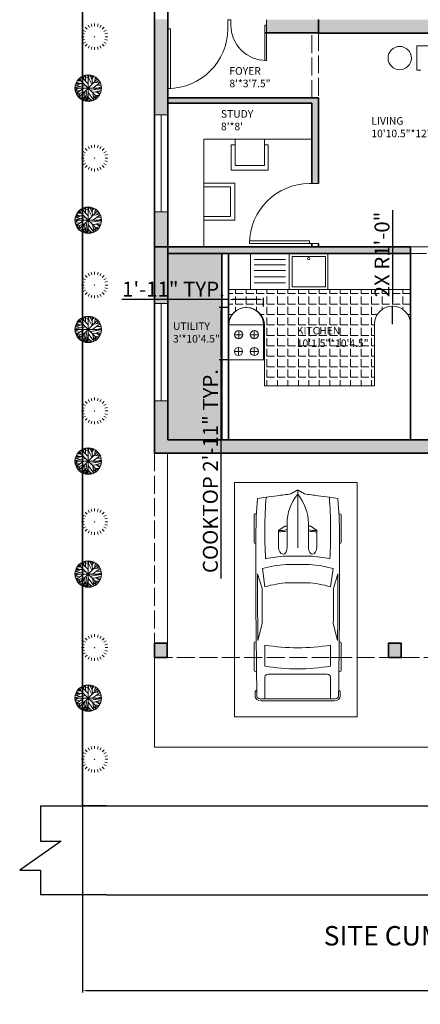
# Model space of a CAD drawing. Units: inches. Extents: x 2852 to 3654, y 1718 to 3031.
# Tile 1 of 5: x 2852 to 3120, y 1718 to 2376. Entities that reach past the tile are written whole.
import ezdxf

# ---------------------------------------------------------------- set-up
doc = ezdxf.new("R2010")
doc.units = ezdxf.units.IN
doc.linetypes.add('ACAD_ISO02W100', pattern=[15, 12, -3])
for name, color, linetype, lineweight in [('A-ANNO-DIMS', 2, 'Continuous', 18), ('A-ANNO-TITL', 7, 'Continuous', 35), ('A-AREA-IDEN', 7, 'Continuous', 18), ('A-COLS', 7, 'Continuous', 35), ('A-COLS-PATT', 8, 'Continuous', 13), ('A-DOOR', 140, 'Continuous', 18), ('A-EQPM', 210, 'Continuous', 18), ('A-FLOR-CASE', 210, 'Continuous', 18), ('A-FLOR-FIXT', 9, 'Continuous', 18), ('A-FLOR-PATT', 52, 'Continuous', 13), ('A-ROOF-OVHD', 140, 'ACAD_ISO02W100', 18), ('A-WALL-OVHD', 140, 'ACAD_ISO02W100', 18), ('A-WALL-PATT', 12, 'Continuous', 13), ('C-PKNG', 8, 'Continuous', 18), ('C-PKNG-VEHI', 140, 'Continuous', 13), ('C-PROP', 7, 'Continuous', 35), ('C-ROAD', 7, 'Continuous', 25), ('fur', 210, 'Continuous', 18), ('tree', 74, 'Continuous', 13), ('wall', 12, 'Continuous', 35), ('window', 140, 'Continuous', 18)]:
    doc.layers.add(name, color=color, linetype=linetype, lineweight=lineweight)
doc.styles.get("Standard").update_dxf_attribs({"font": 'arial.ttf'})
doc.dimstyles.new('ISO-25', dxfattribs={"dimtxt": 10, "dimasz": 2.5, "dimexe": 1.25, "dimexo": 0.625, "dimtad": 1, "dimdec": 0, "dimlunit": 4, "dimtxsty": 'Standard', "dimcen": 2.5, "dimadec": 0, "dimazin": 0, "dimtfac": 1, "dimtdec": 0, "dimtmove": 0, "dimatfit": 3, "dimfxl": 1, "dimarcsym": 0})
pattern_1 = [(0, (0, 0), (0, 6.985), [5.08, -1.905]), (90, (0, 0), (-6.985, 4e-16), [5.08, -1.905])]

# ---------------------------------------------------------------- blocks, each defined once
blk = doc.blocks.new('*U2')
for p, q in [((0, 0), (0, -6)), ((40, 0), (40, -6))]:
    blk.add_line(p, q)
blk.add_lwpolyline([(0, 0), (0, 40), (1.75, 40), (1.75, 0)], close=True)
blk.add_arc((0, 0), 40, 0, 90)
blk = doc.blocks.new('*U6')
for p, q in [((21.1, 37.41), (21.1, 36.83)), ((46.55, 38.89), (22.35, 38.89)), ((47.8, 37.39), (47.8, 37.41)), ((87.99, 31.87), (74.76, 35.92)), ((134.31, 35.6), (119.29, 31.78)), ((135.45, 37.07), (135.45, 37.41)), ((136.7, 38.89), (160.9, 38.89)), ((162.15, 37.41), (162.15, 36.77)), ((70.03, 31.54), (86.41, 29.35)), ((138.42, 29.35), (157.25, 29.35)), ((186.47, 29.35), (167.01, 29.35)), ((186.47, -33.5), (186.47, 33.5)), ((188.4, -32.76), (188.4, 32.76)), ((164.52, 26.39), (164.52, -26.39)), ((29.77, 9.51), (51.68, 9.51)), ((32.12, 9.51), (32.12, 11.15)), ((32.27, 11.63), (36.13, 17.17)), ((36.13, 17.17), (50.94, 17.17)), ((58.92, -10.77), (58.92, 10.77)), ((66.55, -10.53), (66.55, 10.53)), ((186.47, -10.53), (186.47, 10.53)), ((3.27, 6.13), (0.1, 0.41)), ((82.74, 8.5), (82.74, -8.5)), ((0, 0), (51.68, 0)), ((0.1, -0.41), (3.27, -6.13)), ((29.77, -9.51), (51.68, -9.51)), ((32.12, -9.51), (32.12, -11.15)), ((32.27, -11.63), (36.13, -17.17)), ((36.13, -17.17), (50.94, -17.17)), ((86.41, -29.35), (70.03, -31.54)), ((87.99, -31.87), (74.76, -35.92)), ((134.31, -35.6), (119.29, -31.78)), ((157.25, -29.35), (138.42, -29.35)), ((167.01, -29.35), (186.47, -29.35)), ((21.1, -37.41), (21.1, -36.83)), ((46.55, -38.89), (22.35, -38.89)), ((47.8, -37.39), (47.8, -37.41)), ((135.45, -37.07), (135.45, -37.41)), ((136.7, -38.89), (160.9, -38.89)), ((162.15, -37.41), (162.15, -36.77))]:
    blk.add_line(p, q)
for centre, major_axis, ratio, start_param, end_param in [((266.03, -27.52), (0, 313.31), 0.842304, 1.367076, 1.39176), ((41.19, -490.86), (0, 528.23), 0.842304, 0.00281, 0.075598), ((22.35, 37.41), (0, -1.48), 0.842304, 3.141593, 4.712389), ((64.48, -10555.62), (0, 10593.03), 0.842304, -0.013397, 0.002797), ((46.55, 37.41), (0, 1.48), 0.842304, -1.570796, 0), ((64.48, -10555.62), (0, -10591.55), 0.842304, 3.133765, 3.140441), ((136.7, 37.41), (0, -1.48), 0.842304, 3.141593, 4.712389), ((160.9, 37.41), (0, 1.48), 0.842304, -1.570796, 0), ((180.63, 35.84), (0, 2.22), 0.842304, -0.013017, 1.249894), ((64.48, -10556.36), (0, 10595.31), 0.842304, -0.013397, -0.013017), ((183.98, 33.5), (0, -2.96), 0.842304, 1.570796, 3.128196), ((183.98, 32.76), (0, -5.25), 0.842304, 1.570796, 3.128196), ((259.18, -27.52), (0, -305.3), 0.842304, 4.528606, 4.561838), ((37.47, -593.96), (0, -623.33), 0.842304, 3.096046, 3.200911), ((134.4, 5.39), (0, -89.78), 0.842304, 4.449482, 4.652344), ((135.29, 5.39), (0, 81.77), 0.842304, 1.245306, 1.50788), ((149.6, 2.8), (0, -79.58), 0.842304, 4.372215, 4.640744), ((95.79, -3666.35), (0, -3698.24), 0.842304, 3.134049, 3.144098), ((17.08, 0), (0, 147.02), 0.842304, 4.511394, 4.913384), ((35.91, 0), (0, 147.02), 0.842304, 4.511394, 4.913384), ((167.01, 26.39), (0, 2.96), 0.842304, 0, 1.570796), ((-204.49, 52.4), (0, -250.96), 0.842304, 1.385369, 1.434372), ((29.77, -46.66), (0, 56.17), 0.842304, 0, 0.590319), ((32.75, 11.15), (0, 0.74), 0.842304, 0.879714, 1.570796), ((13.04, 17.01), (0, 27.42), 0.842304, 4.435146, 4.718221), ((14.2, 17.01), (0, 27.42), 0.842304, 4.435146, 4.718221), ((50.79, 13.34), (6.34, -0.36), 0.603834, -1.395552, 1.581315), ((0.62, 0), (0, -0.74), 0.842304, 4.131459, 5.293319), ((-204.49, -52.4), (0, 250.96), 0.842304, -1.434372, -1.385369), ((29.77, 46.66), (0, 56.17), 0.842304, 2.551274, 3.141593), ((149.6, -2.8), (0, -79.58), 0.842304, -1.499151, -1.230623), ((32.75, -11.15), (0, -0.74), 0.842304, 4.712389, 5.403472), ((13.04, -17.01), (0, -27.42), 0.842304, 1.564964, 1.848039), ((14.2, -17.01), (0, -27.42), 0.842304, 1.564964, 1.848039), ((134.4, -5.39), (0, -89.78), 0.842304, -1.510751, -1.307889), ((135.29, -5.39), (0, -81.77), 0.842304, -1.50788, -1.245306), ((259.18, 27.52), (0, 305.3), 0.842304, 1.721348, 1.754579), ((167.01, -26.39), (0, -2.96), 0.842304, 4.712389, 6.283185), ((266.03, 27.52), (0, 313.31), 0.842304, 1.749832, 1.774517), ((37.47, 593.96), (0, -623.33), 0.842304, -0.059319, 0.045547), ((95.79, 3666.35), (0, -3698.24), 0.842304, -0.002505, 0.007544), ((183.98, -33.5), (0, 2.96), 0.842304, 3.15499, 4.712389), ((183.98, -32.76), (0, -5.25), 0.842304, 0.013397, 1.570796), ((41.19, 490.86), (0, -528.23), 0.842304, -0.075598, -0.00281), ((22.35, -37.41), (0, 1.48), 0.842304, 1.570796, 3.141593), ((64.48, 10555.62), (0, 10593.03), 0.842304, 3.138796, 3.15499), ((46.55, -37.41), (0, -1.48), 0.842304, 0, 1.570796), ((64.48, 10555.62), (0, -10591.55), 0.842304, 0.001152, 0.007828), ((136.7, -37.41), (0, -1.48), 0.842304, -1.570796, 0), ((160.9, -37.41), (0, 1.48), 0.842304, 3.141593, 4.712389), ((180.63, -35.84), (0, -2.22), 0.842304, -1.249894, 0.013017), ((64.48, 10556.36), (0, 10595.31), 0.842304, 3.15461, 3.15499)]:
    blk.add_ellipse(centre, major_axis=major_axis, ratio=ratio, start_param=start_param, end_param=end_param)
at = {"extrusion": (0, 0, -1)}
blk.add_ellipse((50.79, -13.34), major_axis=(6.34, 0.36), ratio=0.603834, start_param=-1.395552, end_param=1.581315, dxfattribs=at)
blk = doc.blocks.new('*U10')
for p, q in [((-40.1797, 44.558), (-36.4825, 43.2038)), ((-37.0107, 47.0408), (-35.25, 35.5298)), ((-32.6092, 50.4264), (-23.2782, 23.5674)), ((-31.2008, 51.1035), (-0.2149, 20.1818)), ((-26.4472, 46.5894), (-26.2712, 53.8116)), ((-22.0458, 42.0753), (-16.5881, 57.6486)), ((-21.1656, 55.8436), (-0.0388, 45.0094)), ((-12.5388, 54.9406), (-7.9613, 59.4546)), ((-12.3627, 32.1443), (-12.5388, 58.7776)), ((-5.3205, 59.6806), (16.5105, 16.7963)), ((2.426, 54.9406), (-1.4472, 59.9056)), ((0, 59.9996), (0, -60)), ((0.4894, 48.6208), (3.6584, 59.6806)), ((18.2711, 35.5298), (5.419, 59.6806)), ((9.8203, 51.5549), (12.8133, 58.5516)), ((19.6795, 19.5047), (16.3344, 57.6486)), ((17.0387, 51.1035), (23.2006, 55.1666)), ((17.7429, 43.6552), (25.4894, 54.2636)), ((31.6513, 50.8778), (30.2429, 30.5643)), ((31.1232, 42.5267), (35.8767, 48.1693)), ((-59.7219, 2.8025), (-12.0106, 12.0565)), ((-32.2571, 20.6333), (-59.1937, 9.348)), ((-58.6656, 12.7336), (-35.9543, 7.5424)), ((-57.081, 17.9248), (-47.0458, 14.7649)), ((-56.0247, 20.859), (-20.8134, 20.859)), ((-54.7923, 24.4702), (-47.75, 21.0847)), ((-54.6162, -24.7335), (-20.2853, 0.0941)), ((-53.2078, 27.4044), (-40.1797, 20.859)), ((-49.8627, 32.8214), (-32.7853, 32.8214)), ((-45.8134, 38.2383), (-40.5318, 33.0471)), ((-43.8768, 36.4326), (-44.405, 40.2696)), ((42, 42), (-42, -42)), ((42, -42), (-42, 42)), ((54.3626, 25.3731), (20.9119, 0.3198)), ((23.3767, 23.3417), (53.3063, 27.4044)), ((29.3626, -6.6771), (59.4682, 7.091)), ((36.2288, 25.1474), (48.9049, 35.0784)), ((37.1091, 37.1098), (46.6161, 37.5612)), ((38.5175, 13.4107), (58.2359, 13.6364)), ((-60, 0), (60, 0)), ((-59.7219, -4.8714), (-54.2641, -6.6771)), ((-45.2853, -0.1316), (-59.0177, -10.0627)), ((-58.4895, -12.3197), (-36.4825, -11.6426)), ((-57.081, -18.4138), (-45.2853, -17.9624)), ((-52.6797, -18.188), (-55.4966, -22.0251)), ((-53.2078, -27.442), (-16.7641, -16.6081)), ((-38.9472, -29.0219), (-51.4472, -30.6018)), ((-47.2219, -19.3166), (-50.2148, -26.3135)), ((-46.5177, -30.1504), (-49.5106, -33.536)), ((-32.4331, -32.4075), (-48.1021, -35.5674)), ((-43.7008, -34.6645), (-46.6937, -37.373)), ((-35.9543, -22.4765), (-44.0529, -40.5329)), ((-24.6867, -37.8244), (-38.7712, -45.7241)), ((-26.2712, -43.9185), (-34.7219, -48.6583)), ((-19.9331, -20.2194), (-28.5599, -52.721)), ((-14.6515, -36.2445), (-27.6797, -52.9467)), ((-14.8275, -15.0282), (-14.6515, -57.6865)), ((-14.6515, -32.1818), (-3.912, -59.4922)), ((-10.074, -10.0627), (-2.5036, -59.7178)), ((-6.2008, -36.2445), (17.919, -57.0094)), ((-0.0388, -19.0909), (25.8415, -53.8495)), ((9.2922, -9.1598), (59.6443, -2.8401)), ((18.6232, -18.6394), (26.7218, -53.3981)), ((18.7992, -18.6394), (57.3556, -17.2853)), ((22.8485, -36.4702), (35.3485, -48.4326)), ((26.3697, -18.4138), (58.9401, -9.8369)), ((30.419, -30.1504), (32.3556, -50.0125)), ((31.4753, -31.279), (49.6091, -33.3103)), ((38.1654, -18.188), (52.426, -29.0219)), ((41.5105, -32.6332), (46.088, -38.0501)), ((45.9119, -24.0564), (55.595, -22.2508)), ((-14.6515, -47.3041), (-25.0388, -54.3009)), ((-21.5177, -45.4984), (-19.9331, -56.1065)), ((-8.4895, -47.5298), (-11.4825, -58.5893)), ((-6.3768, -52.721), (-9.3698, -58.815)), ((8.4119, -53.1724), (3.8344, -59.4922)), ((5.9471, -46.6269), (10.5246, -58.5893)), ((24.7852, -44.8213), (23.0246, -54.978))]:
    blk.add_line(p, q)
blk.add_circle((0, 0), 60)
blk = doc.blocks.new('*U9')
for p, q in [((-25.024, 42.079), (-31.077, 52.563)), ((-13.435, 46.72), (-16.606, 58.557)), ((-1.077, 60.601), (-1.077, 48.601)), ((11.28, 46.72), (14.452, 58.557)), ((22.87, 42.079), (28.923, 52.563)), ((-61.077, 0.601), (-49.077, 0.601)), ((-47.5, 13.04), (-59.033, 16.131)), ((-42.564, 24.554), (-53.039, 30.601)), ((-34.93, 34.454), (-43.503, 43.028)), ((32.776, 34.454), (41.349, 43.028)), ((40.409, 24.554), (50.884, 30.601)), ((45.346, 13.04), (56.878, 16.131)), ((58.923, 0.601), (46.923, 0.601)), ((-47.5, -11.837), (-59.033, -14.928)), ((-42.564, -23.351), (-53.039, -29.399)), ((-34.93, -33.251), (-43.503, -41.825)), ((-25.024, -40.876), (-31.077, -51.36)), ((22.87, -40.876), (28.923, -51.36)), ((32.776, -33.251), (41.349, -41.825)), ((40.409, -23.351), (50.884, -29.399)), ((45.346, -11.837), (56.878, -14.928)), ((-13.435, -45.517), (-16.606, -57.354)), ((-1.077, -59.399), (-1.077, -47.399)), ((11.28, -45.517), (14.452, -57.354))]:
    blk.add_line(p, q)
blk.add_lwpolyline([(-1.908, 0.978), (-2.67, -0.978), (0, 0)], close=True)
blk = doc.blocks.new('COOKTOP-4-BURNER')
for p, q in [((8.84, 29.44), (3.38, 29.44)), ((6.11, 32.18), (6.11, 26.71)), ((6.11, 26.71), (6.11, 29.44)), ((6.11, 29.44), (8.84, 29.44)), ((19.4, 29.44), (13.94, 29.44)), ((16.67, 32.18), (16.67, 26.71)), ((16.67, 26.71), (16.67, 29.44)), ((16.67, 29.44), (19.4, 29.44)), ((6.11, 20.96), (6.11, 15.5)), ((16.52, 20.96), (16.52, 15.5)), ((8.84, 18.23), (3.38, 18.23)), ((6.11, 15.5), (6.11, 18.23)), ((6.11, 18.23), (8.84, 18.23)), ((19.25, 18.23), (13.79, 18.23)), ((16.52, 15.5), (16.52, 18.23)), ((16.52, 18.23), (19.25, 18.23))]:
    blk.add_line(p, q)
blk.add_lwpolyline([(0, 35.06), (23.09, 35.06), (23.09, 11.55), (0, 11.55)], close=True)
for centre in [(6.11, 29.44), (16.67, 29.44), (6.11, 18.23), (16.52, 18.23)]:
    blk.add_circle(centre, 2.73)
blk.add_arc((11.55, 11.55), 11.55, 180, 0)
blk = doc.blocks.new('ROAD-BREAK')
for p, q in [((13.81, 59.39), (13.81, 35.82)), ((27.65, 35.82), (12.74, 25.36)), ((13.81, 35.82), (27.65, 35.82)), ((12.74, 25.36), (0, 16.42)), ((0, 16.42), (13.81, 16.42)), ((13.81, 16.42), (13.81, 0))]:
    blk.add_line(p, q)
blk = doc.blocks.new('PARKING-STALL')
blk.add_lwpolyline([(0, 156.52), (82.03, 156.52), (82.03, 0), (0, 0)], close=True)
blk = doc.blocks.new('*D37')
at = {"layer": 'A-ANNO-DIMS', "color": 0, "lineweight": -2, "transparency": 16777216}
for p, q in [((2991.43, 2184.07), (2985.55, 2184.07)), ((2986.8, 2181.57), (2986.8, 2151.51)), ((2991.43, 2149.01), (2985.55, 2149.01)), ((2986.8, 2149.01), (2986.8, 2002.92))]:
    blk.add_line(p, q, dxfattribs=at)
at = {"layer": 'A-ANNO-DIMS', "color": 0, "lineweight": 100, "transparency": 16777216}
for points in [[(2986.38, 2181.57), (2987.22, 2181.57), (2986.8, 2184.07)], [(2986.38, 2151.51), (2987.22, 2151.51), (2986.8, 2149.01)]]:
    blk.add_solid(points, dxfattribs=at)
at = {"layer": 'Defpoints', "color": 0, "lineweight": 100, "transparency": 16777216}
for p in [(2992.06, 2184.07), (2986.8, 2149.01), (2992.06, 2149.01)]:
    blk.add_point(p, dxfattribs=at)
at = {"layer": 'A-ANNO-DIMS', "color": 0, "transparency": 16777216, "insert": (2981, 2074.71), "char_height": 10, "attachment_point": 5, "rotation": 90}
blk.add_mtext('COOKTOP 2\'-11" TYP.', dxfattribs=at)
blk = doc.blocks.new('*D38')
at = {"layer": 'A-ANNO-DIMS', "color": 0, "lineweight": -2, "transparency": 16777216}
for p, q in [((2992.06, 2189.33), (2920.53, 2189.33)), ((2992.06, 2184.69), (2992.06, 2190.58)), ((3012.65, 2189.33), (2994.56, 2189.33)), ((3015.15, 2184.69), (3015.15, 2190.58))]:
    blk.add_line(p, q, dxfattribs=at)
at = {"layer": 'A-ANNO-DIMS', "color": 0, "lineweight": 100, "transparency": 16777216}
for points in [[(2994.56, 2189.74), (2994.56, 2188.91), (2992.06, 2189.33)], [(3012.65, 2189.74), (3012.65, 2188.91), (3015.15, 2189.33)]]:
    blk.add_solid(points, dxfattribs=at)
at = {"layer": 'Defpoints', "color": 0, "lineweight": 100, "transparency": 16777216}
for p in [(2992.06, 2189.33), (2992.06, 2184.07), (3015.15, 2184.07)]:
    blk.add_point(p, dxfattribs=at)
at = {"layer": 'A-ANNO-DIMS', "color": 0, "transparency": 16777216, "insert": (2955.04, 2194.98), "char_height": 10, "attachment_point": 5}
blk.add_mtext('1\'-11" TYP.', dxfattribs=at)
blk = doc.blocks.new('*D39')
at = {"layer": 'A-ANNO-DIMS', "color": 0, "lineweight": -2, "transparency": 16777216}
for p, q in [((2894.37, 1850.19), (2894.37, 1726.13)), ((3510.95, 1850.19), (3510.95, 1726.13)), ((2896.87, 1727.38), (3508.45, 1727.38))]:
    blk.add_line(p, q, dxfattribs=at)
at = {"layer": 'A-ANNO-DIMS', "color": 0, "lineweight": 100, "transparency": 16777216}
for points in [[(2896.87, 1727.79), (2896.87, 1726.96), (2894.37, 1727.38)], [(3508.45, 1727.79), (3508.45, 1726.96), (3510.95, 1727.38)]]:
    blk.add_solid(points, dxfattribs=at)
at = {"layer": 'Defpoints', "color": 0, "lineweight": 100, "transparency": 16777216}
for p in [(2894.37, 1850.82), (3510.95, 1850.82), (3510.95, 1727.38)]:
    blk.add_point(p, dxfattribs=at)
at = {"layer": 'A-ANNO-DIMS', "color": 0, "transparency": 16777216, "insert": (3202.66, 1733.17), "char_height": 10, "attachment_point": 5}
blk.add_mtext('51\'-4 1/2"', dxfattribs=at)
blk = doc.blocks.new('*D41')
at = {"layer": 'A-ANNO-DIMS', "color": 0, "lineweight": -2, "transparency": 16777216}
for p, q in [((3101.37, 2248.99), (3101.37, 2187.43)), ((3101.37, 2172.93), (3101.37, 2184.93))]:
    blk.add_line(p, q, dxfattribs=at)
at = {"layer": 'A-ANNO-DIMS', "color": 0, "lineweight": 100, "transparency": 16777216}
blk.add_solid([(3100.95, 2187.43), (3101.78, 2187.43), (3101.37, 2184.93)], dxfattribs=at)
at = {"layer": 'Defpoints', "color": 0, "lineweight": 100, "transparency": 16777216}
for p in [(3101.37, 2184.93), (3101.37, 2172.93)]:
    blk.add_point(p, dxfattribs=at)
at = {"layer": 'A-ANNO-DIMS', "color": 0, "transparency": 16777216, "insert": (3095.64, 2219.46), "char_height": 10, "attachment_point": 5, "rotation": 89.99977}
blk.add_mtext('2X R1\'-0"', dxfattribs=at)

msp = doc.modelspace()

# ---------------------------------------------------------------- hatches: boundary and pattern name
at = {"layer": 'A-COLS-PATT'}
h = msp.add_hatch(color=256, dxfattribs=at)
h.dxf.hatch_style = 1
h.paths.add_polyline_path([(2950.9, 1959.59), (2942.37, 1959.59), (2942.37, 1950.07), (2950.9, 1950.07)])
h.paths.add_polyline_path([(3107.14, 1959.59), (3098.61, 1959.59), (3098.61, 1950.07), (3107.14, 1950.07)])
h.paths.add_polyline_path([(3238.77, 1959.59), (3230.24, 1959.59), (3230.24, 1950.07), (3238.77, 1950.07)])
h.paths.add_polyline_path([(3429.87, 1959.59), (3421.34, 1959.59), (3421.34, 1950.07), (3429.87, 1950.07)])
at = {"layer": 'A-FLOR-PATT'}
h = msp.add_hatch(dxfattribs=at)
h.set_pattern_fill('ANGLE', color=256)
h.set_pattern_definition(pattern_1)
h.paths.add_polyline_path([(3248.45, 2849.58), (3188.45, 2849.58), (3188.45, 2844.77), (3196.45, 2844.77), (3196.45, 2842.27), (3196.95, 2842.27), (3196.95, 2844.27), (3197.95, 2844.27), (3197.95, 2841.27), (3196.45, 2841.27), (3196.45, 2838.27), (3202.45, 2840.27, -0.501317), (3221.31, 2835.31, -0.132891), (3221.31, 2833.22, -0.501323), (3202.45, 2828.27), (3196.45, 2830.27), (3196.45, 2823.77), (3188.45, 2823.77), (3188.45, 2783.69), (3215.78, 2783.69), (3215.78, 2783.73, -0.401453), (3244.71, 2813.96), (3244.71, 2813.99), (3246.03, 2813.99), (3246.03, 2783.69), (3248.45, 2783.69)])
h.paths.add_polyline_path([(3420.95, 2714.69), (3324.42, 2714.69), (3324.42, 2691.18, -1), (3301.33, 2691.18), (3301.33, 2638.19), (3420.95, 2638.19)])
h.paths.add_polyline_path([(3059.57, 2647.05, -0.132891), (3061.66, 2647.05, -0.501323), (3066.62, 2628.19), (3064.62, 2622.19), (3071.12, 2622.19), (3071.12, 2614.19), (3084.95, 2614.19), (3084.95, 2678.69), (3040.14, 2678.69), (3040.14, 2677.19), (3040.14, 2637.19), (3038.39, 2637.19), (3038.39, 2637.23, -0.401453), (3000.14, 2677.19), (3000.14, 2678.69), (2994.25, 2678.69), (2994.25, 2614.19), (3050.12, 2614.19), (3050.12, 2622.19), (3052.62, 2622.19), (3052.62, 2622.69), (3050.62, 2622.69), (3050.62, 2623.69), (3053.62, 2623.69), (3053.62, 2622.19), (3056.62, 2622.19), (3054.62, 2628.19, -0.501317)])
h.paths.add_polyline_path([(3252.95, 2533.88, -0.400409), (3223.79, 2561.89), (3223.76, 2561.89), (3223.76, 2563.17), (3252.95, 2563.17), (3252.95, 2565.48), (3192.95, 2565.48), (3192.95, 2500.92), (3252.95, 2500.92)])
h.paths.add_polyline_path([(3248.45, 2338.72), (3188.45, 2338.72), (3188.45, 2271.48), (3248.45, 2271.48), (3248.45, 2273.69)])
h.paths.add_polyline_path([(3390.34, 2273.69), (3312.95, 2273.69), (3312.95, 2224.19), (3390.34, 2224.19)])
h.paths.add_polyline_path([(3365.33, 2231.19), (3382.33, 2231.19, -0.5), (3383.33, 2230.19), (3383.33, 2226.19, -0.5), (3382.33, 2225.19), (3365.33, 2225.19, -0.5), (3364.33, 2226.19), (3364.33, 2230.19, -0.5)], flags=16)
h.paths.add_polyline_path([(3372.19, 2255.72, -0.215004), (3375.48, 2255.72, -0.48008), (3377.83, 2238.19), (3369.83, 2238.19, -0.48008)], flags=16)
h.paths.add_polyline_path([(2987.37, 2220.07), (2951.37, 2220.07), (2951.37, 2095.57), (2987.37, 2095.57)])
h = msp.add_hatch(dxfattribs=at)
h.set_pattern_fill('ANGLE', color=256)
h.set_pattern_definition(pattern_1)
h.paths.add_polyline_path([(3113.37, 2172.93), (3113.37, 2196.07), (2991.87, 2196.07), (2991.87, 2172.07, -1), (3015.87, 2172.07), (3015.87, 2146.36), (3015.87, 2131.57), (3089.37, 2131.57), (3089.37, 2138.18), (3089.37, 2172.93, -1)])
at = {"layer": 'A-WALL-PATT'}
h = msp.add_hatch(color=256, dxfattribs=at)
h.dxf.hatch_style = 1
h.paths.add_polyline_path([(2952.95, 2875.19), (2957.35, 2875.19), (2957.35, 2877.98), (2957.35, 2884.19), (2943.95, 2884.19), (2942.37, 2884.19), (2942.37, 2849.42), (2952.95, 2849.42)])
h.paths.add_polyline_path([(2952.95, 2706.39), (2952.95, 2749.45), (2942.37, 2749.45), (2942.37, 2667.89), (2952.95, 2667.89), (2952.95, 2678.69), (3000.14, 2678.69), (3000.14, 2683.19), (2952.95, 2683.19)])
h.paths.add_polyline_path([(2951.37, 2609.69), (3089.45, 2609.69), (3089.45, 2683.19), (3089.45, 2685.28), (3084.95, 2685.28), (3084.95, 2683.19), (3084.95, 2614.19), (2952.95, 2614.19), (2952.95, 2625.26), (2942.37, 2625.26), (2942.37, 2588.19), (2951.37, 2588.19)])
h.paths.add_polyline_path([(2951.37, 2506.48), (2951.37, 2523.26), (2942.37, 2523.26), (2942.37, 2465.69), (2951.37, 2465.69), (2951.37, 2466.48)])
h.paths.add_polyline_path([(2951.37, 2367.57), (2951.37, 2370.4), (2951.37, 2376.57), (2942.37, 2376.57), (2942.37, 2312.8), (2951.37, 2312.8), (2951.37, 2320.57), (2951.37, 2324.07)])
h.paths.add_polyline_path([(3051.87, 2324.07), (3047.37, 2324.07), (2951.37, 2324.07), (2951.37, 2320.57), (3047.37, 2320.57), (3047.37, 2296.57), (3047.37, 2266.82), (3051.87, 2266.82)])
h.paths.add_polyline_path([(2951.37, 2224.57), (2942.37, 2224.57), (2942.37, 2186.63), (2951.37, 2186.63), (2951.37, 2220.07)])
h.paths.add_polyline_path([(2951.37, 2247.87), (2942.37, 2247.87), (2942.37, 2224.57), (2951.37, 2224.57)])
h.paths.add_polyline_path([(3113.37, 2224.57), (2951.37, 2224.57), (2951.37, 2220.07), (3113.37, 2220.07)])
h.paths.add_polyline_path([(2951.37, 2121.7), (2942.37, 2121.7), (2942.37, 2086.57), (3113.37, 2086.57), (3147.16, 2086.57), (3147.16, 2095.57), (3113.37, 2095.57), (2951.37, 2095.57)])
h.paths.add_polyline_path([(3429.87, 2224.19), (3276.87, 2224.19), (3276.87, 2219.69), (3420.87, 2219.69), (3420.87, 2182.43), (3429.87, 2182.43)])
h.paths.add_polyline_path([(3276.87, 2175.85), (3272.37, 2175.85), (3272.37, 2095.57), (3240.86, 2095.57), (3240.86, 2086.57), (3276.87, 2086.57)])
h.paths.add_polyline_path([(3276.87, 2224.57), (3234.52, 2224.57), (3234.52, 2220.07), (3272.37, 2220.07), (3272.37, 2215.85), (3276.87, 2215.85)])
h = msp.add_hatch(color=256, dxfattribs=at)
h.dxf.hatch_style = 1
h.paths.add_polyline_path([(3188.45, 2266.98), (3183.95, 2266.98), (3183.95, 2224.57), (3183.95, 2220.07), (3205.81, 2220.07), (3205.81, 2224.57), (3188.45, 2224.57)])
h.paths.add_polyline_path([(3188.45, 2367.48), (3183.95, 2367.48), (3183.95, 2266.98), (3188.45, 2266.98), (3188.45, 2271.48)])
h.paths.add_polyline_path([(3051.87, 2376.48), (3017.1, 2376.48), (3017.1, 2372.85), (3017.1, 2367.57), (3047.37, 2367.57), (3051.87, 2367.57), (3051.87, 2372.07)])
h.paths.add_polyline_path([(3197.45, 2376.48), (3197.45, 2460.48), (3225.82, 2460.48), (3225.82, 2469.48), (3188.45, 2469.48), (3188.45, 2376.48), (3051.87, 2376.48), (3051.87, 2372.07), (3051.87, 2367.48), (3197.45, 2367.48)])
h.paths.add_polyline_path([(3257.45, 2410.19), (3257.45, 2469.48), (3247.17, 2469.48), (3247.17, 2460.48), (3248.45, 2460.48), (3248.45, 2376.48), (3218.8, 2376.48), (3218.8, 2367.48), (3257.45, 2367.48)])
h.paths.add_polyline_path([(3257.45, 2367.48), (3252.95, 2367.48), (3252.95, 2278.19), (3257.45, 2278.19)])
h.paths.add_polyline_path([(3420.95, 2278.19), (3308.45, 2278.19), (3308.45, 2273.69), (3420.95, 2273.69)])
h.paths.add_polyline_path([(3257.45, 2527.51), (3257.45, 2533.88), (3252.95, 2533.88), (3252.95, 2469.48), (3257.45, 2469.48)])
h.paths.add_polyline_path([(3257.45, 2609.69), (3259.24, 2609.69), (3259.24, 2614.19), (3252.95, 2614.19), (3227.77, 2614.19), (3227.77, 2611.84), (3227.77, 2609.69), (3252.95, 2609.69), (3252.95, 2563.17), (3253.06, 2563.17), (3257.45, 2563.17)])
h.paths.add_polyline_path([(3196.43, 2614.19), (3188.45, 2614.19), (3188.45, 2569.84), (3188.45, 2469.48), (3192.95, 2469.48), (3192.95, 2565.48), (3252.95, 2565.48), (3252.95, 2569.98), (3192.95, 2569.98), (3192.95, 2609.69), (3196.43, 2609.69), (3196.43, 2611.84)])

# ---------------------------------------------------------------- linework, layer by layer
at = {"layer": 'A-COLS'}
for p, q in [((2942.37, 1959.59), (2942.37, 1950.07)), ((2942.37, 1950.07), (2950.9, 1950.07))]:
    msp.add_line(p, q, dxfattribs=at)
for points in [[(2942.37, 1950.07), (2950.9, 1950.07), (2950.9, 1959.59), (2942.37, 1959.59)], [(3098.61, 1950.07), (3107.14, 1950.07), (3107.14, 1959.59), (3098.61, 1959.59)]]:
    msp.add_lwpolyline(points, close=True, dxfattribs=at)
at = {"layer": 'A-FLOR-CASE'}
for p, q in [((3047.37, 2320.57), (3047.37, 2296.57)), ((2975.37, 2224.57), (2975.37, 2296.57)), ((3047.37, 2296.57), (2975.37, 2296.57)), ((2951.37, 2224.57), (2975.37, 2224.57)), ((2991.87, 2220.07), (2991.87, 2196.07)), ((2991.87, 2196.07), (3113.37, 2196.07)), ((2991.87, 2196.07), (3015.87, 2196.07)), ((2991.87, 2196.07), (2991.87, 2172.07)), ((3113.37, 2196.07), (3089.37, 2196.07)), ((3113.37, 2196.07), (3113.37, 2172.07)), ((3015.87, 2172.07), (3015.87, 2146.36)), ((3089.37, 2172.93), (3089.37, 2138.18)), ((3015.87, 2146.36), (3015.87, 2131.57)), ((3089.37, 2138.18), (3089.37, 2131.57)), ((2991.87, 2095.57), (2991.87, 2131.57)), ((3015.87, 2131.57), (3089.37, 2131.57))]:
    msp.add_line(p, q, dxfattribs=at)
for centre in [(3003.87, 2172.07), (3101.37, 2172.93)]:
    msp.add_arc(centre, 12, 0, 180, dxfattribs=at)
at = {"layer": 'A-FLOR-FIXT'}
for p, q in [((3032.32, 2220.07), (3032.37, 2196.07)), ((3008.97, 2216), (3029.89, 2216)), ((3008.97, 2212.47), (3029.89, 2212.47)), ((3008.97, 2208.72), (3029.89, 2208.72)), ((3008.97, 2204.54), (3029.89, 2204.54)), ((3008.97, 2200.57), (3029.89, 2200.57))]:
    msp.add_line(p, q, dxfattribs=at)
for points in [[(3006.4, 2220.07), (3058.24, 2220.07), (3058.24, 2196.07), (3006.4, 2196.07)], [(3034.29, 2218.15), (3056.71, 2218.15), (3056.71, 2197.78), (3034.29, 2197.78)]]:
    msp.add_lwpolyline(points, close=True, dxfattribs=at)
msp.add_circle((3045.32, 2216.69), 0.817, dxfattribs=at)
at = {"layer": 'A-ROOF-OVHD'}
for p, q in [((2942.37, 2086.57), (2942.37, 1950.07)), ((2942.37, 1950.07), (3429.87, 1950.07))]:
    msp.add_line(p, q, dxfattribs=at)
at = {"layer": 'A-WALL-OVHD'}
msp.add_line((2991.37, 2376.4), (2993.37, 2376.4), dxfattribs=at)
for points in [[(3051.87, 2324.07), (3047.37, 2324.07), (3047.37, 2367.57), (3051.87, 2367.57)], [(3113.37, 2224.57), (3183.95, 2224.57), (3183.95, 2220.07), (3113.37, 2220.07)]]:
    msp.add_lwpolyline(points, close=True, dxfattribs=at)
at = {"layer": 'C-PKNG'}
for p, q in [((2951.02, 2086.57), (2951.02, 1966.37)), ((2951.02, 1966.37), (2951.02, 1959.59)), ((2942.37, 1950.07), (2942.37, 1890.07)), ((3008.96, 1950.07), (3010.43, 1950.07)), ((3059.99, 1950.07), (3067.12, 1950.07)), ((3098.61, 1950.07), (3107.14, 1950.07)), ((2942.37, 1890.07), (3429.87, 1890.07))]:
    msp.add_line(p, q, dxfattribs=at)
at = {"layer": 'C-PROP'}
for p, q in [((2894.37, 1890.07), (2894.37, 2927.69)), ((2894.37, 1890.07), (2894.37, 1850.82)), ((2894.37, 1850.82), (2910.23, 1850.82))]:
    msp.add_line(p, q, dxfattribs=at)
at = {"layer": 'C-ROAD'}
for p, q in [((2866.16, 1850.82), (2910.23, 1850.82)), ((2910.23, 1850.82), (3468.85, 1850.82)), ((2910.23, 1791.43), (2866.16, 1791.43)), ((2910.23, 1791.43), (3468.85, 1791.43))]:
    msp.add_line(p, q, dxfattribs=at)
at = {"layer": 'fur'}
for p, q in [((3117.65, 2342.6), (3117.65, 2358.82)), ((3117.65, 2358.82), (3156.83, 2358.82)), ((3120.33, 2342.6), (3117.65, 2342.6)), ((2996.17, 2292.84), (2993.65, 2292.84)), ((2993.65, 2292.84), (2993.65, 2275.9)), ((3018.41, 2292.84), (3015.91, 2292.84)), ((3018.41, 2275.9), (3018.41, 2292.84)), ((2993.65, 2275.9), (3018.41, 2275.9)), ((2979.1, 2267.16), (2975.37, 2267.16)), ((2996.03, 2267.16), (2979.1, 2267.16)), ((2996.03, 2242.4), (2996.03, 2267.16)), ((2979.1, 2242.4), (2975.37, 2242.4)), ((2979.1, 2242.4), (2996.03, 2242.4))]:
    msp.add_line(p, q, dxfattribs=at)
for points in [[(2996.17, 2296.57), (3015.91, 2296.57), (3015.91, 2278.85), (2996.17, 2278.85)], [(2975.37, 2244.92), (2975.37, 2264.67), (2993.09, 2264.67), (2993.09, 2244.92)]]:
    msp.add_lwpolyline(points, close=True, dxfattribs=at)
msp.add_circle((3106.15, 2350.75), 7.79, dxfattribs=at)
at = {"layer": 'wall'}
for p, q in [((2942.37, 2224.57), (2942.37, 2884.19)), ((2951.37, 2609.69), (2951.37, 2367.57)), ((3051.87, 2372.07), (3051.87, 2376.48)), ((3051.87, 2372.07), (3051.87, 2367.48)), ((2951.37, 2324.07), (2951.37, 2367.57)), ((3016.06, 2367.57), (3047.37, 2367.57)), ((3047.37, 2367.57), (3051.87, 2367.57)), ((3051.87, 2367.48), (3248.45, 2367.48)), ((2951.37, 2324.07), (3047.37, 2324.07)), ((2951.37, 2320.57), (2951.37, 2324.07)), ((3047.37, 2324.07), (3051.87, 2324.07)), ((3051.87, 2324.07), (3051.87, 2266.82)), ((2951.37, 2224.57), (2951.37, 2320.57)), ((2951.37, 2320.57), (3047.37, 2320.57)), ((3047.37, 2320.57), (3047.37, 2266.82)), ((3113.37, 2224.57), (2942.37, 2224.57)), ((2942.37, 2224.57), (2942.37, 2086.57)), ((2951.37, 2220.07), (2951.37, 2224.57)), ((3047.37, 2226.82), (3047.37, 2224.57)), ((3051.87, 2226.82), (3051.87, 2224.57)), ((3113.37, 2224.57), (3113.37, 2095.57)), ((3113.37, 2220.07), (2951.37, 2220.07)), ((2951.37, 2220.07), (2951.37, 2095.57)), ((2987.37, 2220.07), (2987.37, 2095.57)), ((2991.87, 2220.07), (2991.87, 2095.57)), ((3113.37, 2095.57), (3113.37, 2220.07)), ((2951.37, 2095.57), (3113.37, 2095.57)), ((3113.37, 2095.57), (3272.37, 2095.57)), ((2942.37, 2086.57), (3113.37, 2086.57)), ((3113.37, 2086.57), (3276.87, 2086.57))]:
    msp.add_line(p, q, dxfattribs=at)
at = {"layer": 'window'}
for p, q in [((2946.87, 2247.87), (2946.87, 2312.8)), ((2946.87, 2121.7), (2946.87, 2186.63))]:
    msp.add_line(p, q, dxfattribs=at)
for points in [[(2942.37, 2312.8), (2951.37, 2312.8), (2951.37, 2247.87), (2942.37, 2247.87)], [(2942.37, 2186.63), (2951.37, 2186.63), (2951.37, 2121.7), (2942.37, 2121.7)]]:
    msp.add_lwpolyline(points, close=True, dxfattribs=at)

# ---------------------------------------------------------------- block references
at = {"layer": 'A-DOOR', "xscale": -1, "rotation": 180}
msp.add_blockref('*U2', (2951.37, 2370.4), dxfattribs=at)
at = {"layer": 'A-DOOR', "xscale": 0.5931757633417637, "yscale": 0.5931757633417637, "zscale": 0.5931757633417637, "rotation": 180}
msp.add_blockref('*U2', (3017.1, 2372.85), dxfattribs=at)
at = {"layer": 'A-DOOR', "rotation": 90}
msp.add_blockref('*U2', (3045.87, 2226.82), dxfattribs=at)
at = {"layer": 'A-EQPM', "rotation": 180}
msp.add_blockref('COOKTOP-4-BURNER', (3015.15, 2184.07), dxfattribs=at)
at = {"layer": 'C-PKNG'}
msp.add_blockref('PARKING-STALL', (2995.75, 1910.51), dxfattribs=at)
at = {"layer": 'C-PKNG-VEHI', "xscale": 0.7477922120772245, "yscale": 0.7477922120772245, "zscale": 0.7477922120772245, "rotation": 270}
msp.add_blockref('*U6', (3038.04, 2061.92), dxfattribs=at)
at = {"layer": 'C-ROAD'}
msp.add_blockref('ROAD-BREAK', (2852.35, 1791.43), dxfattribs=at)
at = {"layer": 'tree', "xscale": 0.1480989313836924, "yscale": 0.1480989313836924, "zscale": 0.1480989313836924}
for name, p in [('*U9', (2902.57, 2364.95)), ('*U10', (2898.14, 2330.64)), ('*U9', (2902.57, 2283.83)), ('*U10', (2898.14, 2242.32)), ('*U9', (2902.57, 2198.97)), ('*U10', (2898.14, 2169.41)), ('*U9', (2902.57, 2114.8)), ('*U10', (2898.14, 2081.35)), ('*U9', (2902.57, 2040.77)), ('*U10', (2898.14, 2005.87)), ('*U9', (2902.57, 1956.61)), ('*U10', (2898.14, 1922.97)), ('*U9', (2902.57, 1881.94))]:
    msp.add_blockref(name, p, dxfattribs=at)

# ---------------------------------------------------------------- texts
at = {"layer": 'A-ANNO-TITL', "insert": (3055.38, 1770.57), "char_height": 12.998, "attachment_point": 1}
msp.add_mtext_dynamic_manual_height_columns('SITE CUM GROUND FLOOR PLAN', width=2588.4992, gutter_width=64.99, heights=[0], dxfattribs=at)
at = {"layer": 'A-AREA-IDEN', "attachment_point": 1}
for s, insert, char_height in [('FOYER\\P8\'*3\'7.5"', (2992.41, 2344.69), 5.041), ("STUDY\\P8'*8'", (2986.79, 2315.94), 5.041), ('LIVING\\P10\'10.5"*12\'', (3087.23, 2311.26), 5.0412), ('UTILITY\\P3\'*10\'4.5"', (2954.75, 2174.06), 5.041), ('KITCHEN\\P10\'1.5"*10\'4.5"', (3037.46, 2171.07), 5.0412)]:
    msp.add_mtext_dynamic_manual_height_columns(s, width=98.3816, gutter_width=25.21, heights=[0], dxfattribs=dict(at, insert=insert, char_height=char_height))

# ---------------------------------------------------------------- dimensions: what is measured, and where the dimension line sits
at = {"layer": 'A-ANNO-DIMS'}
dim = msp.add_radius_dim(center=(3101.37, 2172.93), mpoint=(3101.37, 2184.93), text='2X <>', dimstyle='ISO-25', override={"dimdec": 1, "dimlfac": 1, "dimrnd": 0, "dimzin": 1, "dimdsep": 46, "dimlunit": 4, "dimfrac": 2}, dxfattribs=at)
dim.commit()
dim.dimension.update_dxf_attribs({"geometry": '*D41', "text_midpoint": (3095.64, 2219.46)})
for base, p1, p2, angle, text, picture, middle in [((2992.06, 2189.33), (3015.15, 2184.07), (2992.06, 2184.07), 180, '<> TYP.', '*D38', (2955.04, 2194.98)), ((2986.8, 2149.01), (2992.06, 2184.07), (2992.06, 2149.01), 270, 'COOKTOP <> TYP.', '*D37', (2981, 2074.71))]:
    dim = msp.add_linear_dim(base=base, p1=p1, p2=p2, angle=angle, text=text, dimstyle='ISO-25', override={"dimdec": 1, "dimlfac": 1, "dimrnd": 0, "dimzin": 1, "dimdsep": 46, "dimlunit": 4, "dimfrac": 2}, dxfattribs=at)
    dim.commit()
    dim.dimension.update_dxf_attribs({"geometry": picture, "text_midpoint": middle})
dim = msp.add_linear_dim(base=(3510.95, 1727.38), p1=(2894.37, 1850.82), p2=(3510.95, 1850.82), dimstyle='ISO-25', override={"dimdec": 1, "dimlfac": 1, "dimrnd": 0, "dimzin": 1, "dimdsep": 46, "dimlunit": 4, "dimfrac": 2}, dxfattribs=at)
dim.commit()
dim.dimension.update_dxf_attribs({"geometry": '*D39', "text_midpoint": (3202.66, 1733.17)})

doc.saveas('drawing.dxf')
